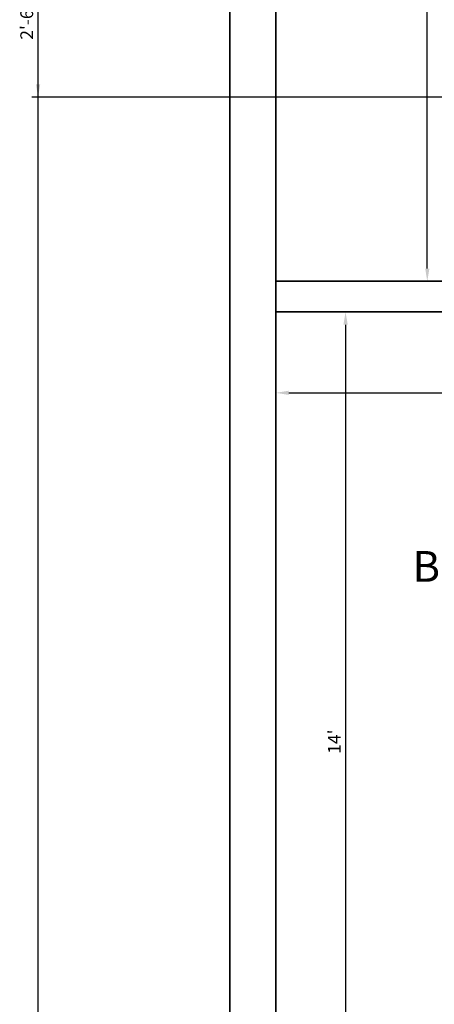
# Model space of a CAD drawing. Units: inches. Extents: x 2025 to 2528, y 1525 to 2336.
# Tile 6 of 18: x 2025 to 2106, y 1974 to 2167. Entities that reach past the tile are written whole.
import ezdxf

# ---------------------------------------------------------------- set-up
doc = ezdxf.new("R2010")
doc.units = ezdxf.units.IN
for name, color, linetype, lineweight in [('A-ANNO-DIMS', 2, 'Continuous', 18), ('A-AREA-IDEN', 7, 'Continuous', 25), ('A-WALL', 7, 'Continuous', 35)]:
    doc.layers.add(name, color=color, linetype=linetype, lineweight=lineweight)
doc.styles.get("Standard").update_dxf_attribs({"font": 'arial.ttf'})
doc.dimstyles.new('Copy of ISO-25', dxfattribs={"dimtxt": 2.5, "dimasz": 2.5, "dimexe": 1.25, "dimexo": 0.625, "dimtad": 1, "dimdec": 1, "dimlunit": 4, "dimtxsty": 'Standard', "dimcen": 2.5, "dimadec": 0, "dimazin": 0, "dimtfac": 1, "dimtdec": 1, "dimtmove": 0, "dimatfit": 3, "dimfxl": 1, "dimarcsym": 0})

# ---------------------------------------------------------------- blocks, each defined once
blk = doc.blocks.new('*D7')
at = {"layer": 'A-ANNO-DIMS', "color": 0, "lineweight": -2, "transparency": 16777216}
for p, q in [((2075.64, 2283.41), (2105.88, 2283.41)), ((2104.63, 2117.91), (2104.63, 2280.91)), ((2075.64, 2115.41), (2105.88, 2115.41))]:
    blk.add_line(p, q, dxfattribs=at)
at = {"layer": 'A-ANNO-DIMS', "color": 0, "transparency": 16777216}
for points in [[(2104.22, 2280.91), (2105.05, 2280.91), (2104.63, 2283.41)], [(2104.22, 2117.91), (2105.05, 2117.91), (2104.63, 2115.41)]]:
    blk.add_solid(points, dxfattribs=at)
at = {"layer": 'Defpoints', "color": 0, "transparency": 16777216}
for p in [(2075.01, 2283.41), (2104.63, 2283.41), (2075.01, 2115.41)]:
    blk.add_point(p, dxfattribs=at)
at = {"layer": 'A-ANNO-DIMS', "color": 0, "transparency": 16777216, "insert": (2102.75, 2199.41), "char_height": 2.5, "attachment_point": 5, "rotation": 90}
blk.add_mtext("14'", dxfattribs=at)
blk = doc.blocks.new('*D12')
at = {"layer": 'A-ANNO-DIMS', "color": 0, "lineweight": -2, "transparency": 16777216}
for p, q in [((2075.01, 2108.79), (2075.01, 2092.35)), ((2207.01, 2108.79), (2207.01, 2092.35)), ((2077.51, 2093.6), (2204.51, 2093.6))]:
    blk.add_line(p, q, dxfattribs=at)
at = {"layer": 'A-ANNO-DIMS', "color": 0, "transparency": 16777216}
for points in [[(2077.51, 2094.02), (2077.51, 2093.19), (2075.01, 2093.6)], [(2204.51, 2094.02), (2204.51, 2093.19), (2207.01, 2093.6)]]:
    blk.add_solid(points, dxfattribs=at)
at = {"layer": 'Defpoints', "color": 0, "transparency": 16777216}
for p in [(2075.01, 2109.41), (2207.01, 2109.41), (2207.01, 2093.6)]:
    blk.add_point(p, dxfattribs=at)
at = {"layer": 'A-ANNO-DIMS', "color": 0, "transparency": 16777216, "insert": (2141.01, 2095.48), "char_height": 2.5, "attachment_point": 5}
blk.add_mtext("11'", dxfattribs=at)
blk = doc.blocks.new('*D13')
at = {"layer": 'A-ANNO-DIMS', "color": 0, "lineweight": -2, "transparency": 16777216}
for p, q in [((2075.64, 2109.41), (2089.89, 2109.41)), ((2088.64, 2106.91), (2088.64, 1943.91)), ((2075.64, 1941.41), (2089.89, 1941.41))]:
    blk.add_line(p, q, dxfattribs=at)
at = {"layer": 'A-ANNO-DIMS', "color": 0, "transparency": 16777216}
for points in [[(2088.22, 2106.91), (2089.06, 2106.91), (2088.64, 2109.41)], [(2088.22, 1943.91), (2089.06, 1943.91), (2088.64, 1941.41)]]:
    blk.add_solid(points, dxfattribs=at)
at = {"layer": 'Defpoints', "color": 0, "transparency": 16777216}
for p in [(2075.01, 2109.41), (2075.01, 1941.41), (2088.64, 1941.41)]:
    blk.add_point(p, dxfattribs=at)
at = {"layer": 'A-ANNO-DIMS', "color": 0, "transparency": 16777216, "insert": (2086.76, 2025.41), "char_height": 2.5, "attachment_point": 5, "rotation": 90}
blk.add_mtext("14'", dxfattribs=at)
blk = doc.blocks.new('*D77')
at = {"layer": 'A-ANNO-DIMS', "color": 0, "lineweight": -2, "transparency": 16777216}
for p, q in [((2254.39, 2181.41), (2027.21, 2181.41)), ((2028.46, 2153.91), (2028.46, 2178.91)), ((2254.39, 2151.41), (2027.21, 2151.41))]:
    blk.add_line(p, q, dxfattribs=at)
at = {"layer": 'A-ANNO-DIMS', "color": 0, "transparency": 16777216}
for points in [[(2028.05, 2178.91), (2028.88, 2178.91), (2028.46, 2181.41)], [(2028.05, 2153.91), (2028.88, 2153.91), (2028.46, 2151.41)]]:
    blk.add_solid(points, dxfattribs=at)
at = {"layer": 'Defpoints', "color": 0, "transparency": 16777216}
for p in [(2028.46, 2181.41), (2255.01, 2181.41), (2255.01, 2151.41)]:
    blk.add_point(p, dxfattribs=at)
at = {"layer": 'A-ANNO-DIMS', "color": 0, "transparency": 16777216, "insert": (2026.56, 2166.41), "char_height": 2.5, "attachment_point": 5, "rotation": 90}
blk.add_mtext('2\'-6"', dxfattribs=at)
blk = doc.blocks.new('*D80')
at = {"layer": 'A-ANNO-DIMS', "color": 0, "lineweight": -2, "transparency": 16777216}
for p, q in [((2065.39, 2292.41), (2027.21, 2292.41)), ((2028.46, 1566.91), (2028.46, 2289.91)), ((2285.39, 1564.41), (2027.21, 1564.41))]:
    blk.add_line(p, q, dxfattribs=at)
at = {"layer": 'A-ANNO-DIMS', "color": 0, "transparency": 16777216}
for points in [[(2028.05, 2289.91), (2028.88, 2289.91), (2028.46, 2292.41)], [(2028.05, 1566.91), (2028.88, 1566.91), (2028.46, 1564.41)]]:
    blk.add_solid(points, dxfattribs=at)
at = {"layer": 'Defpoints', "color": 0, "transparency": 16777216}
for p in [(2028.46, 2292.41), (2066.01, 2292.41), (2286.01, 1564.41)]:
    blk.add_point(p, dxfattribs=at)
at = {"layer": 'A-ANNO-DIMS', "color": 0, "transparency": 16777216, "insert": (2026.56, 1928.41), "char_height": 2.5, "attachment_point": 5, "rotation": 90}
blk.add_mtext('60\'-8"', dxfattribs=at)

msp = doc.modelspace()

# ---------------------------------------------------------------- linework, layer by layer
at = {"layer": 'A-WALL'}
for p, q in [((2066.01, 2283.41), (2066.01, 2115.41)), ((2075.01, 2283.41), (2075.01, 2115.41)), ((2075.01, 2283.41), (2075.01, 2115.41)), ((2066.01, 2115.41), (2066.01, 2109.41)), ((2075.01, 2115.41), (2075.01, 2109.41)), ((2075.01, 2115.41), (2225.01, 2115.41)), ((2066.01, 2109.41), (2066.01, 1941.41)), ((2075.01, 2109.41), (2075.01, 1941.41)), ((2075.01, 2109.41), (2207.01, 2109.41)), ((2207.01, 2109.41), (2075.01, 2109.41)), ((2075.01, 2109.41), (2207.01, 2109.41))]:
    msp.add_line(p, q, dxfattribs=at)

# ---------------------------------------------------------------- texts
at = {"layer": 'A-AREA-IDEN'}
msp.add_text('BED ROOM 02', height=6, dxfattribs=at).set_placement((2101.75, 2056.67))

# ---------------------------------------------------------------- dimensions: what is measured, and where the dimension line sits
at = {"layer": 'A-ANNO-DIMS'}
for base, p1, p2, override, picture, middle in [((2028.46, 2292.41), (2286.01, 1564.41), (2066.01, 2292.41), {"dimdec": 1, "dimlfac": 1, "dimrnd": 0, "dimzin": 1, "dimdsep": 46, "dimlunit": 4, "dimfrac": 2}, '*D80', (2026.56, 1928.41)), ((2104.63, 2283.41), (2075.01, 2115.41), (2075.01, 2283.41), {"dimclrd": 0, "dimclre": 0, "dimclrt": 0}, '*D7', (2102.75, 2199.41)), ((2028.46, 2181.41), (2255.01, 2151.41), (2255.01, 2181.41), {"dimdec": 1, "dimlfac": 1, "dimrnd": 0, "dimzin": 1, "dimdsep": 46, "dimlunit": 4, "dimfrac": 2}, '*D77', (2026.56, 2166.41)), ((2088.64, 1941.41), (2075.01, 2109.41), (2075.01, 1941.41), {"dimclrd": 0, "dimclre": 0, "dimclrt": 0}, '*D13', (2086.76, 2025.41))]:
    dim = msp.add_linear_dim(base=base, p1=p1, p2=p2, angle=90, dimstyle='Copy of ISO-25', override=override, dxfattribs=at)
    dim.commit()
    dim.dimension.update_dxf_attribs({"geometry": picture, "text_midpoint": middle})
dim = msp.add_linear_dim(base=(2207.01, 2093.6), p1=(2075.01, 2109.41), p2=(2207.01, 2109.41), dimstyle='Copy of ISO-25', override={"dimclrd": 0, "dimclre": 0, "dimclrt": 0}, dxfattribs=at)
dim.commit()
dim.dimension.update_dxf_attribs({"geometry": '*D12', "text_midpoint": (2141.01, 2095.48)})

doc.saveas('drawing.dxf')
